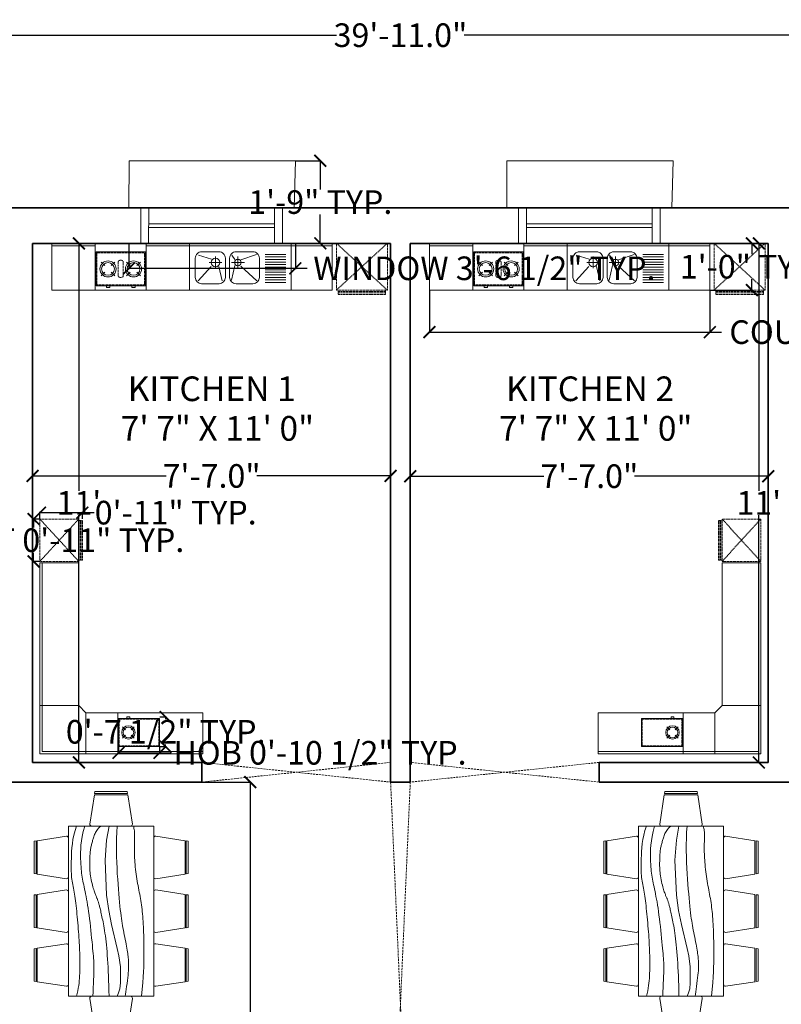
# Model space of a CAD drawing. Units: inches. Extents: x 844 to 2234, y 346 to 1084.
# Tile 92 of 93: x 1840 to 2033, y 828 to 1078. Entities that reach past the tile are written whole.
import ezdxf

# ---------------------------------------------------------------- set-up
doc = ezdxf.new("R2010")
doc.units = ezdxf.units.IN
doc.header["$MEASUREMENT"] = 0
doc.linetypes.add('DASHED', pattern=[0.75, 0.5, -0.25])
doc.linetypes.add('HIDDEN', pattern=[0.375, 0.25, -0.125])
for name, color, linetype, lineweight in [('A-ANNO-DIMS', 2, 'Continuous', 18), ('A-AREA-IDEN', 7, 'Continuous', 18), ('A-EQPM', 42, 'Continuous', 18), ('A-EQPM-HIDN', 42, 'HIDDEN', 13), ('A-FLOR-CASE', 42, 'Continuous', 18), ('A-FLOR-FIXT', 8, 'Continuous', 18), ('A-WALL', 7, 'Continuous', 35), ('A-WALL-OVHD', 7, 'DASHED', 18), ('furniture', 8, 'Continuous', 18), ('windows', 1, 'Continuous', 18)]:
    doc.layers.add(name, color=color, linetype=linetype, lineweight=lineweight)
doc.styles.add('ATTR', font='romans.shx', dxfattribs={"width": 0.8, "height": 0.7})
doc.styles.get("Standard").update_dxf_attribs({"font": 'arial.ttf'})
doc.dimstyles.get("Standard").update_dxf_attribs({"dimtxt": 6, "dimasz": 3, "dimexe": 0.18, "dimexo": 0.0625, "dimgap": 0.09, "dimtad": 0, "dimtih": 1, "dimtoh": 1, "dimdec": 1, "dimzin": 0, "dimdsep": 46, "dimlunit": 3, "dimtxsty": 'Standard', "dimblk": 'ARCHTICK', "dimcen": 0.09, "dimadec": 0, "dimazin": 0, "dimtfac": 1, "dimtdec": 1, "dimtofl": 0, "dimtmove": 0, "dimatfit": 3, "dimfxl": 1, "dimtolj": 1, "dimtzin": 0, "dimarcsym": 0})

# ---------------------------------------------------------------- blocks, each defined once
blk = doc.blocks.new('DIN42X84')
for p, q in [((-34.772, 36.500609), (-37.0377, 21.999999)), ((-34.7681, 36.499999), (-18.2986, 36.499999)), ((-34.5377, 37.999999), (-34.6939, 37.000439)), ((-18.3793, 36.999999), (-34.6911, 36.999999)), ((-34.5377, 37.999999), (-18.5377, 37.999999)), ((-18.3814, 36.999659), (-18.5377, 37.999999)), ((-16.0377, 21.999999), (-18.3032, 36.499269)), ((-8.2343, 36.500609), (-10.5001, 21.999999)), ((-8.2305, 36.499999), (8.2391, 36.499999)), ((-8.0001, 37.999999), (-8.1562, 37.000439)), ((8.1584, 36.999999), (-8.1535, 36.999999)), ((-8.0001, 37.999999), (7.9999, 37.999999)), ((8.1562, 36.999659), (7.9999, 37.999999)), ((10.4999, 21.999999), (8.2344, 36.499269)), ((16.0376, 21.999999), (18.3031, 36.499269)), ((34.768, 36.499999), (18.2985, 36.499999)), ((18.3792, 36.999999), (34.691, 36.999999)), ((18.3813, 36.999659), (18.5376, 37.999999)), ((34.5376, 37.999999), (18.5376, 37.999999)), ((34.5376, 37.999999), (34.6938, 37.000439)), ((34.7719, 36.500609), (37.0376, 21.999999)), ((-43, 10.499989), (-57.4993, 8.234489)), ((43, 10.499989), (57.4992, 8.234489)), ((-57.9997, 8.156299), (-59, 7.999989)), ((-59, -8.000011), (-59, 7.999989)), ((-58, 8.158429), (-58, -8.153391)), ((-57.5, -8.230411), (-57.5, 8.239139)), ((57.5, -8.230411), (57.5, 8.239139)), ((57.9996, 8.156299), (59, 7.999989)), ((58, 8.158429), (58, -8.153391)), ((59, -8.000011), (59, 7.999989)), ((-59, -8.000011), (-58.0005, -8.156181)), ((-57.5007, -8.234271), (-43, -10.500011)), ((57.5006, -8.234271), (43, -10.500011)), ((59, -8.000011), (58.0004, -8.156181)), ((-42, -21.000001), (42, -21.000001)), ((-34.772, -36.50061), (-37.0377, -22.000001)), ((-16.0377, -22.000001), (-18.3032, -36.499267)), ((-8.2343, -36.50061), (-10.5001, -22.000001)), ((10.4999, -22.000001), (8.2344, -36.499267)), ((16.0376, -22.000001), (18.3031, -36.499267)), ((34.7719, -36.50061), (37.0376, -22.000001)), ((-34.7681, -36.499999), (-18.2986, -36.499999)), ((-34.5377, -37.999999), (-34.6939, -37.000442)), ((-18.3793, -36.999999), (-34.6911, -36.999999)), ((-34.5377, -37.999999), (-18.5377, -37.999999)), ((-18.3814, -36.999664), (-18.5377, -37.999999)), ((-8.2305, -36.499999), (8.2391, -36.499999)), ((-8.0001, -37.999999), (-8.1562, -37.000442)), ((8.1584, -36.999999), (-8.1535, -36.999999)), ((-8.0001, -37.999999), (7.9999, -37.999999)), ((8.1562, -36.999664), (7.9999, -37.999999)), ((34.768, -36.499999), (18.2985, -36.499999)), ((18.3792, -36.999999), (34.691, -36.999999)), ((18.3813, -36.999664), (18.5376, -37.999999)), ((34.5376, -37.999999), (18.5376, -37.999999)), ((34.5376, -37.999999), (34.6938, -37.000442))]:
    blk.add_line(p, q)
for points in [[(-42, -21.000001), (-42, 20.999989), (42, 20.999989), (42, -21.000001)], [(-42, 16.999989), (-40.5974, 16.672209), (-39.2569, 16.395939), (-37.9668, 16.166109), (-36.7153, 15.977689), (-35.4906, 15.825599), (-34.281, 15.704799), (-33.0745, 15.610229), (-31.8595, 15.536839), (-30.6267, 15.480229), (-29.3778, 15.438619), (-28.117, 15.410889), (-26.8486, 15.395929), (-25.5767, 15.392599), (-24.3058, 15.399809), (-23.0399, 15.416409), (-21.7833, 15.441309), (-20.5384, 15.473619), (-19.2994, 15.513549), (-18.0587, 15.561549), (-16.8087, 15.618049), (-15.5417, 15.683499), (-14.25, 15.758369), (-12.9261, 15.843079), (-11.5622, 15.938089), (-10.1541, 16.043559), (-8.7108, 16.158419), (-7.2445, 16.281349), (-5.7675, 16.410999), (-4.2923, 16.546019), (-2.8311, 16.685069), (-1.3963, 16.826809), (0, 16.969889), (1.3474, 17.113339), (2.6447, 17.257689), (3.8928, 17.403829), (5.0924, 17.552659), (6.2444, 17.705069), (7.3498, 17.861959), (8.4092, 18.024219), (9.4237, 18.192759), (10.3952, 18.367629), (11.3311, 18.545639), (12.2397, 18.722759), (13.1297, 18.894949), (14.0095, 19.058179), (14.8876, 19.208429), (15.7725, 19.341659), (16.6727, 19.453839), (17.5977, 19.541909), (18.5617, 19.606689), (19.5795, 19.649979), (20.6664, 19.673569), (21.8374, 19.679239), (23.1076, 19.668789), (24.492, 19.644009), (26.0058, 19.606689), (27.6589, 19.554579), (29.4413, 19.469229), (31.3377, 19.328169), (33.3331, 19.108889), (35.4121, 18.788919), (37.5598, 18.345779), (39.7608, 17.756959), (42, 16.999989)], [(42, 12.999999), (39.3635, 13.704689), (36.9303, 14.232849), (34.6868, 14.608169), (32.6195, 14.854319), (30.7149, 14.994989), (28.9596, 15.053859), (27.34, 15.054629), (25.8427, 15.020959), (24.4543, 14.972439), (23.1628, 14.912279), (21.9562, 14.839589), (20.8227, 14.753449), (19.7504, 14.652989), (18.7273, 14.537299), (17.7416, 14.405489), (16.7814, 14.256669), (15.8348, 14.090369), (14.8899, 13.907959), (13.9348, 13.711209), (12.9575, 13.501929), (11.9464, 13.281899), (10.8893, 13.052909), (9.7745, 12.816759), (8.59, 12.575229), (7.3261, 12.330049), (5.9815, 12.082619), (4.557, 11.834299), (3.0536, 11.586429), (1.472, 11.340349), (-0.187, 11.097409), (-1.9223, 10.858939), (-3.7333, 10.626289), (-5.6141, 10.400739), (-7.539, 10.183249), (-9.4776, 9.974709), (-11.3991, 9.776019), (-13.2731, 9.588079), (-15.0689, 9.411789), (-16.756, 9.248039), (-18.3038, 9.097709), (-19.6928, 8.961719), (-20.9483, 8.840959), (-22.1065, 8.736319), (-23.2037, 8.648689), (-24.2763, 8.578979), (-25.3606, 8.528079), (-26.4928, 8.496879), (-27.7094, 8.486279), (-29.0411, 8.496689), (-30.4965, 8.526549), (-32.0787, 8.573829), (-33.7908, 8.636479), (-35.6359, 8.712459), (-37.6171, 8.799739), (-39.7374, 8.896259), (-42, 8.999999)], [(-42, 0.999999), (-39.2567, 1.059739), (-36.6668, 1.127399), (-34.2177, 1.203389), (-31.897, 1.288099), (-29.6923, 1.381949), (-27.5912, 1.485329), (-25.5812, 1.598659), (-23.65, 1.722319), (-21.7874, 1.856519), (-19.9935, 2.000569), (-18.2704, 2.153579), (-16.6207, 2.314649), (-15.0465, 2.482879), (-13.5503, 2.657379), (-12.1344, 2.837259), (-10.8011, 3.021619), (-9.5514, 3.209479), (-8.3812, 3.399579), (-7.2848, 3.590579), (-6.2569, 3.781129), (-5.2918, 3.969889), (-4.384, 4.155509), (-3.5281, 4.336659), (-2.7184, 4.511979), (-1.9505, 4.680359), (-1.2233, 4.841579), (-0.5369, 4.995629), (0.1087, 5.142519), (0.7135, 5.282239), (1.2776, 5.414799), (1.8009, 5.540189), (2.2834, 5.658409), (2.7259, 5.769699), (3.1323, 5.875159), (3.5073, 5.976139), (3.8555, 6.073989), (4.1816, 6.170049), (4.4904, 6.265659), (4.7863, 6.362169), (5.0742, 6.460919), (5.3584, 6.563099), (5.6417, 6.669299), (5.9267, 6.779989), (6.216, 6.895609), (6.512, 7.016589), (6.8174, 7.143399), (7.1347, 7.276479), (7.4664, 7.416279), (7.8159, 7.563169), (8.1896, 7.717219), (8.5948, 7.878439), (9.0386, 8.046819), (9.5282, 8.222369), (10.071, 8.405079), (10.674, 8.594959), (11.3446, 8.791999), (12.0866, 8.995459), (12.8902, 9.201609), (13.7421, 9.405969), (14.6294, 9.604059), (15.5387, 9.791399), (16.4569, 9.963509), (17.3709, 10.115919), (18.2674, 10.244149), (19.1361, 10.344989), (19.9772, 10.420299), (20.7936, 10.473209), (21.5884, 10.506879), (22.3645, 10.524419), (23.1248, 10.528969), (23.8725, 10.523669), (24.6103, 10.511649), (25.3403, 10.495379), (26.0601, 10.474629), (26.7663, 10.448509), (27.4556, 10.416119), (28.1244, 10.376559), (28.7695, 10.328939), (29.3873, 10.272359), (29.9746, 10.205939), (30.5293, 10.129059), (31.0552, 10.042329), (31.5572, 9.946639), (32.0406, 9.842899), (32.5104, 9.731989), (32.9716, 9.614799), (33.4295, 9.492249), (33.8891, 9.365219), (34.3546, 9.234229), (34.8266, 9.098309), (35.3051, 8.956129), (35.7897, 8.806329), (36.2802, 8.647569), (36.7765, 8.478519), (37.2783, 8.297819), (37.7854, 8.104139), (38.2976, 7.894309), (38.8146, 7.657969), (39.3361, 7.382899), (39.8617, 7.056919), (40.3912, 6.667829), (40.9243, 6.203449), (41.4607, 5.651569), (42, 4.999999)], [(42, 0.999999), (35.1214, 2.295539), (25.1178, 2.983399), (7.9376, 2.295539), (0.3261, 1.149099), (-6.6329, -0.226611), (-18.3763, -2.978061), (-22.0733, -3.895201), (-27.5101, -4.583071), (-32.9468, -4.583071), (-35.339, -4.583071), (-38.3836, -4.353771), (-40.3408, -3.665921), (-42, -3.000001)], [(42, -3.000001), (38.9344, -2.781351), (35.8829, -2.650251), (32.8567, -2.595491), (29.8672, -2.605821), (26.9257, -2.670031), (24.0436, -2.776881), (21.2323, -2.915141), (18.5031, -3.073591), (15.8668, -3.242611), (13.3327, -3.419021), (10.9095, -3.601241), (8.6059, -3.787731), (6.4305, -3.976901), (4.3921, -4.167191), (2.4994, -4.357031), (0.7611, -4.544851), (-0.8196, -4.729651), (-2.2614, -4.912671), (-3.5885, -5.095681), (-4.8252, -5.280481), (-5.9956, -5.468861), (-7.1239, -5.662621), (-8.2344, -5.863551), (-9.3513, -6.073431), (-10.4925, -6.293091), (-11.6511, -6.519461), (-12.814, -6.748531), (-13.968, -6.976251), (-15.0999, -7.198591), (-16.1965, -7.411531), (-17.2447, -7.611041), (-18.2313, -7.793081), (-19.1472, -7.954521), (-19.9994, -8.095811), (-20.7989, -8.218291), (-21.5568, -8.323311), (-22.2841, -8.412201), (-22.9919, -8.486311), (-23.6912, -8.546991), (-24.393, -8.595581), (-25.1087, -8.632751), (-25.8513, -8.656491), (-26.6337, -8.664101), (-27.4693, -8.652901), (-28.3711, -8.620211), (-29.3523, -8.563341), (-30.4262, -8.479601), (-31.6057, -8.366301), (-32.8956, -8.222561), (-34.2657, -8.054761), (-35.6772, -7.871051), (-37.0913, -7.679611), (-38.4695, -7.488621), (-39.7728, -7.306241), (-40.9626, -7.140641), (-42, -7.000001)], [(-42, -15.000001), (-38.4722, -15.350691), (-35.3039, -15.623741), (-32.4544, -15.828971), (-29.8831, -15.976191), (-27.5493, -16.075201), (-25.4123, -16.135831), (-23.4313, -16.167881), (-21.5659, -16.181151), (-19.7812, -16.183881), (-18.0665, -16.177871), (-16.4173, -16.163351), (-14.8288, -16.140551), (-13.2964, -16.109691), (-11.8154, -16.070991), (-10.3811, -16.024671), (-8.9888, -15.970971), (-7.6345, -15.909991), (-6.3163, -15.841401), (-5.0329, -15.764751), (-3.7831, -15.679591), (-2.5656, -15.585471), (-1.3791, -15.481951), (-0.2223, -15.368571), (0.9061, -15.244901), (2.0079, -15.110631), (3.0876, -14.966051), (4.1503, -14.811631), (5.2011, -14.647801), (6.2451, -14.475011), (7.2875, -14.293721), (8.3332, -14.104361), (9.3874, -13.907391), (10.4544, -13.703711), (11.5349, -13.495991), (12.6291, -13.287381), (13.7368, -13.081011), (14.8581, -12.880011), (15.9931, -12.687521), (17.1416, -12.506671), (18.3037, -12.340601), (19.4778, -12.191771), (20.6562, -12.059961), (21.8295, -11.944271), (22.9884, -11.843811), (24.1234, -11.757681), (25.2254, -11.684981), (26.2848, -11.624831), (27.2925, -11.576311), (28.2412, -11.538551), (29.1325, -11.510631), (29.9703, -11.491671), (30.7584, -11.480781), (31.5007, -11.477041), (32.2009, -11.479581), (32.8628, -11.487491), (33.4904, -11.499881), (34.0874, -11.515741), (34.6576, -11.533621), (35.2049, -11.551941), (35.733, -11.569151), (36.2459, -11.583661), (36.7473, -11.593931), (37.2411, -11.598371), (37.7311, -11.595421), (38.2211, -11.583281), (38.7152, -11.559251), (39.2177, -11.520361), (39.7326, -11.463671), (40.2641, -11.386241), (40.8164, -11.285111), (41.3937, -11.157351), (42, -11.000001)]]:
    blk.add_lwpolyline(points)
for centre, start, end in [((-36.0377, 21.999999), 180, 270), ((-17.0377, 21.999999), 270, 0), ((-9.5001, 21.999999), 180, 270), ((9.4999, 21.999999), 270, 0), ((17.0376, 21.999999), 180, 270), ((36.0376, 21.999999), 270, 0), ((-43, 9.499989), 0.00000068, 90), ((43, 9.499989), 90, 180), ((-43, -9.500011), 270, 0.00000068), ((43, -9.500011), 180, 270), ((-36.0377, -22.000001), 90, 180), ((-17.0377, -22.000001), 0, 90), ((-9.5001, -22.000001), 90, 180), ((9.4999, -22.000001), 0, 90), ((17.0376, -22.000001), 90, 180), ((36.0376, -22.000001), 0, 90)]:
    blk.add_arc(centre, 1, start, end)
at = {"style": 'ATTR', "width": 0.8, "flags": 9}
blk.add_attdef('ESTCODE', (0, 0), '', height=0.7, dxfattribs=at)
blk = doc.blocks.new('_ArchTick')
at = {"color": 0, "linetype": 'ByBlock', "const_width": 0.15}
blk.add_lwpolyline([(-0.5, -0.5), (0.5, 0.5)], dxfattribs=at)
blk = doc.blocks.new('*D90')
at = {"layer": 'A-ANNO-DIMS', "color": 0, "lineweight": -2, "transparency": 16777216}
for p, q in [((1843.1, 962.31), (1877.06, 962.31)), ((1843.1, 962.25), (1843.1, 962.13)), ((1934.1, 962.31), (1900.13, 962.31)), ((1934.1, 962.37), (1934.1, 962.49))]:
    blk.add_line(p, q, dxfattribs=at)
at = {"layer": 'Defpoints', "color": 0, "transparency": 16777216}
for p in [(1843.1, 962.31), (1934.1, 962.31), (1934.1, 962.31)]:
    blk.add_point(p, dxfattribs=at)
at = {"layer": 'A-ANNO-DIMS', "color": 0, "lineweight": -2, "transparency": 16777216, "xscale": 3, "yscale": 3, "zscale": 3, "rotation": 180}
blk.add_blockref('_ArchTick', (1843.1, 962.31), dxfattribs=at)
at = {"layer": 'A-ANNO-DIMS', "color": 0, "lineweight": -2, "transparency": 16777216, "xscale": 3, "yscale": 3, "zscale": 3}
blk.add_blockref('_ArchTick', (1934.1, 962.31), dxfattribs=at)
at = {"layer": 'A-ANNO-DIMS', "color": 0, "transparency": 16777216, "insert": (1888.6, 962.31), "char_height": 6, "attachment_point": 5}
blk.add_mtext('\\A1;7\'-7.0"', dxfattribs=at)
blk = doc.blocks.new('*D57')
at = {"layer": 'A-ANNO-DIMS', "color": 0, "lineweight": -2, "transparency": 16777216}
for p, q in [((1846.19, 1021.46), (1855.04, 1021.46)), ((1854.86, 1021.46), (1854.86, 958.56)), ((1854.86, 889.46), (1854.86, 952.35)), ((1846.19, 889.46), (1855.04, 889.46))]:
    blk.add_line(p, q, dxfattribs=at)
at = {"layer": 'Defpoints', "color": 0, "transparency": 16777216}
for p in [(1846.12, 1021.46), (1846.12, 889.46), (1854.86, 889.46)]:
    blk.add_point(p, dxfattribs=at)
at = {"layer": 'A-ANNO-DIMS', "color": 0, "lineweight": -2, "transparency": 16777216, "xscale": 3, "yscale": 3, "zscale": 3}
for p, rotation in [((1854.86, 1021.46), 90), ((1854.86, 889.46), 270)]:
    blk.add_blockref('_ArchTick', p, dxfattribs=dict(at, rotation=rotation))
at = {"layer": 'A-ANNO-DIMS', "color": 0, "transparency": 16777216, "insert": (1854.86, 955.46), "char_height": 6, "attachment_point": 5}
blk.add_mtext("\\A1;11'", dxfattribs=at)
blk = doc.blocks.new('*D58')
at = {"layer": 'A-ANNO-DIMS', "color": 0, "lineweight": -2, "transparency": 16777216}
for p, q in [((2029.69, 1021.46), (2027.51, 1021.46)), ((2027.69, 1021.46), (2027.69, 958.56)), ((2027.69, 889.46), (2027.69, 952.35)), ((2029.69, 889.46), (2027.51, 889.46))]:
    blk.add_line(p, q, dxfattribs=at)
at = {"layer": 'Defpoints', "color": 0, "transparency": 16777216}
for p in [(2029.76, 1021.46), (2027.69, 889.46), (2029.76, 889.46)]:
    blk.add_point(p, dxfattribs=at)
at = {"layer": 'A-ANNO-DIMS', "color": 0, "lineweight": -2, "transparency": 16777216, "xscale": 3, "yscale": 3, "zscale": 3}
for p, rotation in [((2027.69, 1021.46), 90), ((2027.69, 889.46), 270)]:
    blk.add_blockref('_ArchTick', p, dxfattribs=dict(at, rotation=rotation))
at = {"layer": 'A-ANNO-DIMS', "color": 0, "transparency": 16777216, "insert": (2027.69, 955.46), "char_height": 6, "attachment_point": 5}
blk.add_mtext("\\A1;11'", dxfattribs=at)
blk = doc.blocks.new('*D59')
at = {"layer": 'A-ANNO-DIMS', "color": 0, "lineweight": -2, "transparency": 16777216}
for p, q in [((1939.1, 962.31), (1939.1, 962.43)), ((1939.1, 962.25), (1973.06, 962.25)), ((2030.1, 962.25), (1996.13, 962.25)), ((2030.1, 962.31), (2030.1, 962.43))]:
    blk.add_line(p, q, dxfattribs=at)
at = {"layer": 'Defpoints', "color": 0, "transparency": 16777216}
for p in [(1939.1, 962.25), (2030.1, 962.25), (2030.1, 962.25)]:
    blk.add_point(p, dxfattribs=at)
at = {"layer": 'A-ANNO-DIMS', "color": 0, "lineweight": -2, "transparency": 16777216, "xscale": 3, "yscale": 3, "zscale": 3, "rotation": 180}
blk.add_blockref('_ArchTick', (1939.1, 962.25), dxfattribs=at)
at = {"layer": 'A-ANNO-DIMS', "color": 0, "lineweight": -2, "transparency": 16777216, "xscale": 3, "yscale": 3, "zscale": 3}
blk.add_blockref('_ArchTick', (2030.1, 962.25), dxfattribs=at)
at = {"layer": 'A-ANNO-DIMS', "color": 0, "transparency": 16777216, "insert": (1984.6, 962.25), "char_height": 6, "attachment_point": 5}
blk.add_mtext('\\A1;7\'-7.0"', dxfattribs=at)
blk = doc.blocks.new('*D85')
at = {"layer": 'A-ANNO-DIMS', "color": 0, "lineweight": -2, "transparency": 16777216}
for p, q in [((1886.16, 884.46), (1898.6, 884.46)), ((1898.42, 884.46), (1898.42, 763.55)), ((1898.42, 636.33), (1898.42, 757.24)), ((1886.16, 636.33), (1898.6, 636.33))]:
    blk.add_line(p, q, dxfattribs=at)
at = {"layer": 'Defpoints', "color": 0, "transparency": 16777216}
for p in [(1886.1, 884.46), (1886.1, 636.33), (1898.42, 636.33)]:
    blk.add_point(p, dxfattribs=at)
at = {"layer": 'A-ANNO-DIMS', "color": 0, "lineweight": -2, "transparency": 16777216, "xscale": 3, "yscale": 3, "zscale": 3}
for p, rotation in [((1898.42, 884.46), 90), ((1898.42, 636.33), 270)]:
    blk.add_blockref('_ArchTick', p, dxfattribs=dict(at, rotation=rotation))
at = {"layer": 'A-ANNO-DIMS', "color": 0, "transparency": 16777216, "insert": (1898.42, 760.39), "char_height": 6, "attachment_point": 5}
blk.add_mtext('\\A1;20\'-8.1"', dxfattribs=at)
blk = doc.blocks.new('*D86')
at = {"layer": 'A-ANNO-DIMS', "color": 0, "lineweight": -2, "transparency": 16777216}
for p, q in [((1697.1, 1030.52), (1697.1, 1074.57)), ((1697.1, 1074.39), (1920.38, 1074.39)), ((2176.1, 1074.39), (1952.82, 1074.39)), ((2176.1, 1030.52), (2176.1, 1074.57))]:
    blk.add_line(p, q, dxfattribs=at)
at = {"layer": 'Defpoints', "color": 0, "transparency": 16777216}
for p in [(2176.1, 1074.39), (1697.1, 1030.46), (2176.1, 1030.46)]:
    blk.add_point(p, dxfattribs=at)
at = {"layer": 'A-ANNO-DIMS', "color": 0, "lineweight": -2, "transparency": 16777216, "xscale": 3, "yscale": 3, "zscale": 3, "rotation": 180}
blk.add_blockref('_ArchTick', (1697.1, 1074.39), dxfattribs=at)
at = {"layer": 'A-ANNO-DIMS', "color": 0, "lineweight": -2, "transparency": 16777216, "xscale": 3, "yscale": 3, "zscale": 3}
blk.add_blockref('_ArchTick', (2176.1, 1074.39), dxfattribs=at)
at = {"layer": 'A-ANNO-DIMS', "color": 0, "transparency": 16777216, "insert": (1936.6, 1074.39), "char_height": 6, "attachment_point": 5}
blk.add_mtext('\\A1;39\'-11.0"', dxfattribs=at)
blk = doc.blocks.new('WIN-36IN')
for p, q in [((0, 9), (0, 21)), ((0, 21), (42.29, 21)), ((42, 9), (42.29, 21)), ((3, 9), (0, 9)), ((39, 9), (3, 9)), ((3, 9), (3, 0)), ((5, 9), (5, 0)), ((37, 0), (37, 9)), ((39, 0), (39, 9)), ((39, 9), (42, 9)), ((5, 5), (37, 5)), ((5, 4), (37, 4)), ((3, 0), (39, 0))]:
    blk.add_line(p, q)
blk = doc.blocks.new('KITCHEN-TALL-UNIT')
for p, q in [((12.96, 1.08), (0, 12.96)), ((0, 1.08), (12.96, 12.96)), ((0.43, 0.73), (12.53, 0.73)), ((0.43, 0.37), (12.53, 0.37))]:
    blk.add_line(p, q)
blk.add_lwpolyline([(0, 1.08), (0, 12.96), (12.96, 12.96), (12.96, 1.08)], close=True)
blk.add_lwpolyline([(0.43, 1.08), (0.43, 0), (12.53, 0), (12.53, 1.08)])
blk = doc.blocks.new('KITCHEN-TALL-UNIT-COMPACT')
for p, q in [((9.89, 0), (0, 10.79)), ((9.89, 10.79), (0, 0)), ((10.18, 0.36), (10.18, 10.43)), ((10.48, 0.36), (10.48, 10.43))]:
    blk.add_line(p, q)
blk.add_lwpolyline([(9.89, 0), (0, 0), (0, 10.79), (9.89, 10.79)], close=True)
blk.add_lwpolyline([(9.89, 0.36), (10.79, 0.36), (10.79, 10.43), (9.89, 10.43)])
blk = doc.blocks.new('KITCHEN-COUNTER-LINEAR')
for p, q in [((0, 11.88), (34.99, 11.88)), ((0, 11.88), (0, 0)), ((0, 11.23), (11.08, 11.23)), ((11.08, 11.88), (11.08, 0)), ((24.04, 11.88), (24.04, 0)), ((24.04, 11.23), (34.99, 11.23)), ((34.99, 11.23), (60.91, 11.23)), ((60.91, 11.88), (71.28, 11.88)), ((60.91, 11.23), (71.28, 11.23)), ((71.28, 11.88), (71.28, 0)), ((0, 0), (34.99, 0)), ((60.91, 0), (71.28, 0))]:
    blk.add_line(p, q)
blk = doc.blocks.new('KITCHEN-COUNTER-L')
for p, q in [((0, 0), (0, 48.56)), ((0, 48.56), (9.89, 48.56)), ((0.54, 0.54), (0.54, 48.56)), ((9.89, 12.23), (9.89, 48.56)), ((9.89, 12.23), (0, 12.23)), ((11.69, 10.43), (9.89, 12.23)), ((11.69, 10.43), (11.69, 0)), ((11.69, 10.43), (41.36, 10.43)), ((19.78, 0), (19.78, 10.43)), ((41.36, 0), (41.36, 10.43)), ((0.54, 0.54), (41.36, 0.54)), ((0, 0), (41.36, 0)), ((0, 0), (9.89, 0))]:
    blk.add_line(p, q)
blk = doc.blocks.new('HOB-2-BURNER')
for p, q in [((1.27, 6.49), (2.18, 5.57)), ((3.86, 5.57), (4.78, 6.49)), ((7.75, 6.49), (8.66, 5.57)), ((10.34, 5.57), (11.26, 6.49)), ((1.27, 2.97), (2.18, 3.89)), ((3.86, 3.89), (4.78, 2.97)), ((7.75, 2.97), (8.66, 3.89)), ((10.34, 3.89), (11.26, 2.97))]:
    blk.add_line(p, q)
blk.add_lwpolyline([(0, 9.07), (0, 0.43), (12.53, 0.43), (12.53, 9.07)], close=True)
for points in [[(2.59, 0.43), (2.59, 0), (3.46, 0), (3.46, 0.45)], [(9.07, 0.43), (9.07, 0), (9.94, 0), (9.94, 0.45)]]:
    blk.add_lwpolyline(points)
for centre, radius in [((3.02, 4.73), 2.05), ((3.02, 4.73), 1.62), ((9.5, 4.73), 2.05), ((9.5, 4.73), 1.62)]:
    blk.add_circle(centre, radius)
blk = doc.blocks.new('HOB-1-BURNER')
for p, q in [((1.82, 4.31), (1.06, 5.08)), ((3.98, 5.08), (3.22, 4.31)), ((1.82, 2.92), (1.06, 2.15)), ((3.98, 2.15), (3.22, 2.92))]:
    blk.add_line(p, q)
blk.add_lwpolyline([(2.88, 7.19), (2.88, 7.55), (2.16, 7.55), (2.16, 7.18)])
blk.add_lwpolyline([(10.43, 0), (10.43, 7.19), (0, 7.19), (0, 0)], close=True)
for radius in [1.71, 1.35]:
    blk.add_circle((2.52, 3.61), radius)
blk = doc.blocks.new('SINK-DOUBLE-DRAINBOARD')
for p, q in [((5.62, 7.84), (2.31, 8.86)), ((6.65, 5.57), (6.65, 8.58)), ((11.53, 7.78), (10.82, 8.86)), ((12.33, 5.55), (12.33, 8.55)), ((13.11, 7.71), (17.09, 9.07)), ((19.31, 9.07), (24.52, 9.07)), ((19.31, 8.42), (24.52, 8.42)), ((19.31, 7.78), (24.52, 7.78)), ((2.23, 2.35), (5.55, 5.96)), ((5.05, 7.02), (8.29, 7.02)), ((8.36, 2.35), (7.5, 5.96)), ((10.74, 7), (13.98, 7)), ((11.53, 6.26), (10.74, 2.51)), ((13.11, 6.11), (17.15, 2.35)), ((19.31, 7.13), (24.52, 7.13)), ((19.31, 6.48), (24.52, 6.48)), ((19.31, 5.83), (24.52, 5.83)), ((19.31, 5.18), (24.52, 5.18)), ((19.31, 4.54), (24.52, 4.54)), ((19.31, 3.89), (24.52, 3.89)), ((19.31, 3.24), (24.52, 3.24)), ((19.31, 2.59), (24.52, 2.59)), ((19.31, 1.94), (24.52, 1.94))]:
    blk.add_line(p, q)
blk.add_lwpolyline([(0, 0), (25.92, 0), (25.92, 11.88), (0, 11.88)], close=True)
for points in [[(1.51, 8.1), (1.51, 3.24, 0.414214), (3.13, 1.62), (7.54, 1.62, 0.414214), (9.16, 3.24), (9.16, 8.1, 0.414214), (7.54, 9.72), (3.13, 9.72, 0.414214)], [(10.24, 8.1), (10.24, 3.24, 0.414214), (11.86, 1.62), (16.18, 1.62, 0.414214), (17.8, 3.24), (17.8, 8.1, 0.414214), (16.18, 9.72), (11.86, 9.72, 0.414214)]]:
    blk.add_lwpolyline(points, format="xyb", close=True)
for centre, radius in [((6.65, 7.02), 1.08), ((12.33, 7), 0.81)]:
    blk.add_circle(centre, radius)
blk = doc.blocks.new('*D123')
at = {"layer": 'A-ANNO-DIMS', "color": 0, "lineweight": -2, "transparency": 16777216}
for p, q in [((1867.6, 1021.4), (1867.6, 1014.93)), ((1909.89, 1021.39), (1909.89, 1014.93)), ((1867.6, 1015.11), (1909.89, 1015.11)), ((1909.89, 1015.11), (1912.89, 1015.11))]:
    blk.add_line(p, q, dxfattribs=at)
at = {"layer": 'Defpoints', "color": 0, "transparency": 16777216}
for p in [(1867.6, 1021.46), (1909.89, 1021.45), (1909.89, 1015.11)]:
    blk.add_point(p, dxfattribs=at)
at = {"layer": 'A-ANNO-DIMS', "color": 0, "lineweight": -2, "transparency": 16777216, "xscale": 3, "yscale": 3, "zscale": 3}
for p, rotation in [((1867.6, 1015.11), 179.9931124012453), ((1909.89, 1015.11), 359.9931124012453)]:
    blk.add_blockref('_ArchTick', p, dxfattribs=dict(at, rotation=rotation))
at = {"layer": 'A-ANNO-DIMS', "color": 0, "transparency": 16777216, "insert": (1957.93, 1015.11), "char_height": 6, "attachment_point": 5}
blk.add_mtext('\\A1;WINDOW 3\'-6 1/2" TYP.', dxfattribs=at)
blk = doc.blocks.new('*D124')
at = {"layer": 'A-ANNO-DIMS', "color": 0, "lineweight": -2, "transparency": 16777216}
for p, q in [((1909.95, 1042.45), (1916.41, 1042.45)), ((1916.23, 1042.45), (1916.23, 1035.11)), ((1916.23, 1021.45), (1916.23, 1028.8)), ((1909.95, 1021.45), (1916.41, 1021.45))]:
    blk.add_line(p, q, dxfattribs=at)
at = {"layer": 'Defpoints', "color": 0, "transparency": 16777216}
for p in [(1909.89, 1042.45), (1916.23, 1042.45), (1909.89, 1021.45)]:
    blk.add_point(p, dxfattribs=at)
at = {"layer": 'A-ANNO-DIMS', "color": 0, "lineweight": -2, "transparency": 16777216, "xscale": 3, "yscale": 3, "zscale": 3}
for p, rotation in [((1916.23, 1042.45), 89.99311240124487), ((1916.23, 1021.45), 269.9931124012449)]:
    blk.add_blockref('_ArchTick', p, dxfattribs=dict(at, rotation=rotation))
at = {"layer": 'A-ANNO-DIMS', "color": 0, "transparency": 16777216, "insert": (1916.23, 1031.95), "char_height": 6, "attachment_point": 5}
blk.add_mtext('\\A1;1\'-9" TYP.', dxfattribs=at)
blk = doc.blocks.new('*D127')
at = {"layer": 'A-ANNO-DIMS', "color": 0, "lineweight": -2, "transparency": 16777216}
for p, q in [((1844.9, 951.36), (1843.17, 951.36)), ((1843.35, 951.36), (1843.35, 949.16)), ((1843.35, 940.57), (1843.35, 942.78)), ((1844.9, 940.57), (1843.17, 940.57))]:
    blk.add_line(p, q, dxfattribs=at)
at = {"layer": 'Defpoints', "color": 0, "transparency": 16777216}
for p in [(1843.35, 951.36), (1844.97, 951.36), (1844.97, 940.57)]:
    blk.add_point(p, dxfattribs=at)
at = {"layer": 'A-ANNO-DIMS', "color": 0, "lineweight": -2, "transparency": 16777216, "xscale": 3, "yscale": 3, "zscale": 3}
for p, rotation in [((1843.35, 951.36), 90), ((1843.35, 940.57), 270)]:
    blk.add_blockref('_ArchTick', p, dxfattribs=dict(at, rotation=rotation))
at = {"layer": 'A-ANNO-DIMS', "color": 0, "transparency": 16777216, "insert": (1843.35, 945.97), "char_height": 6, "attachment_point": 5}
blk.add_mtext('\\A1;CABINET 0\'-11" TYP.', dxfattribs=at)
blk = doc.blocks.new('*D128')
at = {"layer": 'A-ANNO-DIMS', "color": 0, "lineweight": -2, "transparency": 16777216}
for p, q in [((1844.97, 951.43), (1844.97, 953.16)), ((1844.97, 952.98), (1855.76, 952.98)), ((1855.76, 951.43), (1855.76, 953.16)), ((1855.76, 952.98), (1858.76, 952.98))]:
    blk.add_line(p, q, dxfattribs=at)
at = {"layer": 'Defpoints', "color": 0, "transparency": 16777216}
for p in [(1855.76, 952.98), (1844.97, 951.36), (1855.76, 951.36)]:
    blk.add_point(p, dxfattribs=at)
at = {"layer": 'A-ANNO-DIMS', "color": 0, "lineweight": -2, "transparency": 16777216, "xscale": 3, "yscale": 3, "zscale": 3, "rotation": 180}
blk.add_blockref('_ArchTick', (1844.97, 952.98), dxfattribs=at)
at = {"layer": 'A-ANNO-DIMS', "color": 0, "lineweight": -2, "transparency": 16777216, "xscale": 3, "yscale": 3, "zscale": 3}
blk.add_blockref('_ArchTick', (1855.76, 952.98), dxfattribs=at)
at = {"layer": 'A-ANNO-DIMS', "color": 0, "transparency": 16777216, "insert": (1879.47, 952.98), "char_height": 6, "attachment_point": 5}
blk.add_mtext('\\A1;0\'-11" TYP.', dxfattribs=at)
blk = doc.blocks.new('*D129')
at = {"layer": 'A-ANNO-DIMS', "color": 0, "lineweight": -2, "transparency": 16777216}
for p, q in [((1943.95, 1009.51), (1943.95, 998.7)), ((2015.23, 1009.51), (2015.23, 998.7)), ((1943.95, 998.88), (2015.23, 998.88)), ((2015.23, 998.88), (2018.23, 998.88))]:
    blk.add_line(p, q, dxfattribs=at)
at = {"layer": 'Defpoints', "color": 0, "transparency": 16777216}
for p in [(1943.95, 1009.57), (2015.23, 1009.57), (2015.23, 998.88)]:
    blk.add_point(p, dxfattribs=at)
at = {"layer": 'A-ANNO-DIMS', "color": 0, "lineweight": -2, "transparency": 16777216, "xscale": 3, "yscale": 3, "zscale": 3, "rotation": 180}
blk.add_blockref('_ArchTick', (1943.95, 998.88), dxfattribs=at)
at = {"layer": 'A-ANNO-DIMS', "color": 0, "lineweight": -2, "transparency": 16777216, "xscale": 3, "yscale": 3, "zscale": 3}
blk.add_blockref('_ArchTick', (2015.23, 998.88), dxfattribs=at)
at = {"layer": 'A-ANNO-DIMS', "color": 0, "transparency": 16777216, "insert": (2067.78, 998.88), "char_height": 6, "attachment_point": 5}
blk.add_mtext('\\A1;COUNTER 5\'-11 1/2" TYP.', dxfattribs=at)
blk = doc.blocks.new('*D130')
at = {"layer": 'A-ANNO-DIMS', "color": 0, "lineweight": -2, "transparency": 16777216}
for p, q in [((2015.29, 1021.46), (2026.1, 1021.46)), ((2025.92, 1021.46), (2025.92, 1018.67)), ((2025.92, 1009.57), (2025.92, 1012.36)), ((2015.29, 1009.57), (2026.1, 1009.57))]:
    blk.add_line(p, q, dxfattribs=at)
at = {"layer": 'Defpoints', "color": 0, "transparency": 16777216}
for p in [(2015.23, 1021.46), (2025.92, 1021.46), (2015.23, 1009.57)]:
    blk.add_point(p, dxfattribs=at)
at = {"layer": 'A-ANNO-DIMS', "color": 0, "lineweight": -2, "transparency": 16777216, "xscale": 3, "yscale": 3, "zscale": 3}
for p, rotation in [((2025.92, 1021.46), 90), ((2025.92, 1009.57), 270)]:
    blk.add_blockref('_ArchTick', p, dxfattribs=dict(at, rotation=rotation))
at = {"layer": 'A-ANNO-DIMS', "color": 0, "transparency": 16777216, "insert": (2025.92, 1015.51), "char_height": 6, "attachment_point": 5}
blk.add_mtext('\\A1;1\'-0" TYP.', dxfattribs=at)
blk = doc.blocks.new('*D135')
at = {"layer": 'A-ANNO-DIMS', "color": 0, "lineweight": -2, "transparency": 16777216}
for p, q in [((1864.93, 893.41), (1864.93, 891.73)), ((1864.93, 891.91), (1875.36, 891.91)), ((1875.36, 893.41), (1875.36, 891.73)), ((1875.36, 891.91), (1878.36, 891.91))]:
    blk.add_line(p, q, dxfattribs=at)
at = {"layer": 'Defpoints', "color": 0, "transparency": 16777216}
for p in [(1864.93, 893.47), (1875.36, 893.47), (1875.36, 891.91)]:
    blk.add_point(p, dxfattribs=at)
at = {"layer": 'A-ANNO-DIMS', "color": 0, "lineweight": -2, "transparency": 16777216, "xscale": 3, "yscale": 3, "zscale": 3, "rotation": 180}
blk.add_blockref('_ArchTick', (1864.93, 891.91), dxfattribs=at)
at = {"layer": 'A-ANNO-DIMS', "color": 0, "lineweight": -2, "transparency": 16777216, "xscale": 3, "yscale": 3, "zscale": 3}
blk.add_blockref('_ArchTick', (1875.36, 891.91), dxfattribs=at)
at = {"layer": 'A-ANNO-DIMS', "color": 0, "transparency": 16777216, "insert": (1916.14, 891.91), "char_height": 6, "attachment_point": 5}
blk.add_mtext('\\A1;HOB 0\'-10 1/2" TYP.', dxfattribs=at)
blk = doc.blocks.new('*D136')
at = {"layer": 'A-ANNO-DIMS', "color": 0, "lineweight": -2, "transparency": 16777216}
for p, q in [((1875.42, 901.03), (1877.1, 901.03)), ((1876.92, 901.03), (1876.92, 900.44)), ((1876.92, 893.47), (1876.92, 894.06)), ((1875.42, 893.47), (1877.1, 893.47))]:
    blk.add_line(p, q, dxfattribs=at)
at = {"layer": 'Defpoints', "color": 0, "transparency": 16777216}
for p in [(1875.36, 901.03), (1876.92, 901.03), (1875.36, 893.47)]:
    blk.add_point(p, dxfattribs=at)
at = {"layer": 'A-ANNO-DIMS', "color": 0, "lineweight": -2, "transparency": 16777216, "xscale": 3, "yscale": 3, "zscale": 3}
for p, rotation in [((1876.92, 901.03), 90), ((1876.92, 893.47), 270)]:
    blk.add_blockref('_ArchTick', p, dxfattribs=dict(at, rotation=rotation))
at = {"layer": 'A-ANNO-DIMS', "color": 0, "transparency": 16777216, "insert": (1876.92, 897.25), "char_height": 6, "attachment_point": 5}
blk.add_mtext('\\A1;0\'-7 1/2" TYP.', dxfattribs=at)

msp = doc.modelspace()

# ---------------------------------------------------------------- linework, layer by layer
at = {"layer": 'A-EQPM-HIDN'}
for points in [[(1859.46, 1019.08), (1859.46, 1010.87), (1871.56, 1010.87), (1871.56, 1019.08)], [(1955.46, 1019.08), (1955.46, 1010.87), (1967.56, 1010.87), (1967.56, 1019.08)], [(1875.18, 893.65), (1875.18, 900.49), (1865.11, 900.49), (1865.11, 893.65)], [(1998.02, 893.65), (1998.02, 900.49), (2008.09, 900.49), (2008.09, 893.65)]]:
    msp.add_lwpolyline(points, close=True, dxfattribs=at)
for points in [[(1864.86, 1016.7), (1864.86, 1013.25, 0.414214), (1865.29, 1012.81), (1865.73, 1012.81, 0.414214), (1866.16, 1013.25), (1866.16, 1016.7, 0.414214), (1865.73, 1017.14), (1865.29, 1017.14, 0.414214)], [(1960.86, 1016.7), (1960.86, 1013.25, 0.414214), (1961.29, 1012.81), (1961.73, 1012.81, 0.414214), (1962.16, 1013.25), (1962.16, 1016.7, 0.414214), (1961.73, 1017.14), (1961.29, 1017.14, 0.414214)]]:
    msp.add_lwpolyline(points, format="xyb", close=True, dxfattribs=at)
at = {"layer": 'A-FLOR-FIXT'}
for p, q in [((1888.56, 1017.42), (1885.25, 1018.43)), ((1888, 1016.6), (1891.24, 1016.6)), ((1889.59, 1015.15), (1889.59, 1018.15)), ((1893.68, 1016.57), (1896.92, 1016.57)), ((1894.48, 1017.35), (1893.76, 1018.43)), ((1895.28, 1015.13), (1895.28, 1018.13)), ((1896.05, 1017.29), (1900.03, 1018.65)), ((1902.25, 1018.65), (1907.46, 1018.65)), ((1902.25, 1018), (1907.46, 1018)), ((1902.25, 1017.35), (1907.46, 1017.35)), ((1902.25, 1016.7), (1907.46, 1016.7)), ((1885.17, 1011.93), (1888.49, 1015.54)), ((1891.3, 1011.93), (1890.44, 1015.54)), ((1894.48, 1015.84), (1893.68, 1012.08)), ((1896.05, 1015.69), (1900.09, 1011.93)), ((1902.25, 1016.05), (1907.46, 1016.05)), ((1902.25, 1015.41), (1907.46, 1015.41)), ((1902.25, 1014.76), (1907.46, 1014.76)), ((1902.25, 1014.11), (1907.46, 1014.11)), ((1902.25, 1013.46), (1907.46, 1013.46)), ((1902.25, 1012.81), (1907.46, 1012.81)), ((1902.25, 1012.17), (1907.46, 1012.17)), ((1902.25, 1011.52), (1907.46, 1011.52))]:
    msp.add_line(p, q, dxfattribs=at)
msp.add_lwpolyline([(1882.94, 1009.57), (1908.86, 1009.57), (1908.86, 1021.46), (1882.94, 1021.46)], close=True, dxfattribs=at)
for points in [[(1884.45, 1017.68), (1884.45, 1012.81, 0.414214), (1886.07, 1011.19), (1890.48, 1011.19, 0.414214), (1892.1, 1012.81), (1892.1, 1017.68, 0.414214), (1890.48, 1019.3), (1886.07, 1019.3, 0.414214)], [(1893.18, 1017.68), (1893.18, 1012.81, 0.414214), (1894.8, 1011.19), (1899.12, 1011.19, 0.414214), (1900.74, 1012.81), (1900.74, 1017.68, 0.414214), (1899.12, 1019.3), (1894.8, 1019.3, 0.414214)]]:
    msp.add_lwpolyline(points, format="xyb", close=True, dxfattribs=at)
for centre, radius in [((1889.59, 1016.6), 1.08), ((1895.28, 1016.57), 0.81)]:
    msp.add_circle(centre, radius, dxfattribs=at)
at = {"layer": 'A-WALL'}
for p, q in [((1697.1, 1030.46), (2176.1, 1030.46)), ((1843.1, 1021.46), (1843.1, 889.46)), ((1843.1, 1021.46), (1934.1, 1021.46)), ((1934.1, 1021.46), (1934.1, 889.46)), ((1939.1, 1021.46), (1939.1, 889.46)), ((1939.1, 1021.46), (2030.1, 1021.46)), ((2030.1, 1021.46), (2030.1, 889.46)), ((1843.1, 889.46), (1886.1, 889.46)), ((1886.1, 889.46), (1886.1, 884.46)), ((1934.1, 889.46), (1934.1, 884.46)), ((1939.1, 889.46), (1939.1, 884.46)), ((1987.1, 889.46), (2030.1, 889.46)), ((1987.1, 889.46), (1987.1, 884.46)), ((1834.1, 884.46), (1886.1, 884.46)), ((1934.1, 884.46), (1939.1, 884.46)), ((1987.1, 884.46), (2039.1, 884.46))]:
    msp.add_line(p, q, dxfattribs=at)
at = {"layer": 'A-WALL-OVHD'}
for p, q in [((1886.1, 889.46), (1934.1, 884.46)), ((1886.1, 884.46), (1934.1, 889.46)), ((1987.1, 889.46), (1939.1, 884.46)), ((1987.1, 884.46), (1939.1, 889.46)), ((1939.1, 771.46), (1934.1, 884.46)), ((1939.1, 884.46), (1934.1, 771.46))]:
    msp.add_line(p, q, dxfattribs=at)

# ---------------------------------------------------------------- block references
at = {"layer": 'A-EQPM'}
for name, p in [('HOB-2-BURNER', (1859.25, 1010.22)), ('HOB-2-BURNER', (1955.25, 1010.22)), ('HOB-1-BURNER', (1864.93, 893.47))]:
    msp.add_blockref(name, p, dxfattribs=at)
at = {"layer": 'A-EQPM', "extrusion": (0, 0, -1), "zscale": -1}
msp.add_blockref('HOB-1-BURNER', (-2008.27, 893.47), dxfattribs=at)
at = {"layer": 'A-EQPM-HIDN'}
for name, p in [('KITCHEN-TALL-UNIT', (1920.31, 1008.49)), ('KITCHEN-TALL-UNIT', (2016.31, 1008.49)), ('KITCHEN-TALL-UNIT-COMPACT', (1844.97, 940.57))]:
    msp.add_blockref(name, p, dxfattribs=at)
at = {"layer": 'A-EQPM-HIDN', "extrusion": (0, 0, -1), "zscale": -1}
msp.add_blockref('KITCHEN-TALL-UNIT-COMPACT', (-2028.23, 940.57), dxfattribs=at)
at = {"layer": 'A-FLOR-CASE'}
for name, p in [('KITCHEN-COUNTER-LINEAR', (1847.95, 1009.57)), ('KITCHEN-COUNTER-LINEAR', (1943.95, 1009.57)), ('KITCHEN-COUNTER-L', (1844.97, 891.68))]:
    msp.add_blockref(name, p, dxfattribs=at)
at = {"layer": 'A-FLOR-CASE', "extrusion": (0, 0, -1), "zscale": -1}
msp.add_blockref('KITCHEN-COUNTER-L', (-2028.23, 891.68), dxfattribs=at)
at = {"layer": 'A-FLOR-FIXT'}
msp.add_blockref('SINK-DOUBLE-DRAINBOARD', (1978.94, 1009.57), dxfattribs=at)
at = {"layer": 'furniture', "xscale": 0.5153672157522483, "yscale": 0.5153672157522483, "zscale": 0.5153672157522483, "rotation": 90}
for p in [(1863.05, 851.63), (2007.91, 851.63)]:
    msp.add_blockref('DIN42X84', p, dxfattribs=at)
at = {"layer": 'windows', "rotation": 359.9931124012453}
for p in [(1867.6, 1021.46), (1963.6, 1021.46)]:
    msp.add_blockref('WIN-36IN', p, dxfattribs=at)

# ---------------------------------------------------------------- texts
at = {"layer": 'A-AREA-IDEN'}
for s, height, p in [('KITCHEN 1', 6.269, (1867.27, 981.34)), ('KITCHEN 2', 6.269, (1963.44, 981.34)), (' 7\' 7" X 11\' 0"', 6.2688, (1863.57, 971.27)), (' 7\' 7" X 11\' 0"', 6.2688, (1959.74, 971.27))]:
    msp.add_text(s, height=height, dxfattribs=at).set_placement(p)

# ---------------------------------------------------------------- dimensions: what is measured, and where the dimension line sits
at = {"layer": 'A-ANNO-DIMS'}
for base, p1, p2, picture, middle in [((2176.1, 1074.39), (1697.1, 1030.46), (2176.1, 1030.46), '*D86', (1936.6, 1074.39)), ((1934.1, 962.31), (1843.1, 962.31), (1934.1, 962.31), '*D90', (1888.6, 962.31)), ((2030.1, 962.25), (1939.1, 962.25), (2030.1, 962.25), '*D59', (1984.6, 962.25))]:
    dim = msp.add_linear_dim(base=base, p1=p1, p2=p2, dimstyle='Standard', override={"dimclrd": 0, "dimclre": 0, "dimclrt": 0}, dxfattribs=at)
    dim.commit()
    dim.dimension.update_dxf_attribs({"geometry": picture, "text_midpoint": middle})
for base, p1, p2, angle, text, picture, middle in [((1916.23, 1042.45), (1909.89, 1021.45), (1909.89, 1042.45), 89.9931, '<> TYP.', '*D124', (1916.23, 1031.95)), ((1909.89, 1015.11), (1867.6, 1021.46), (1909.89, 1021.45), 359.9931, 'WINDOW <> TYP.', '*D123', (1957.93, 1015.11)), ((2025.92, 1021.46), (2015.23, 1009.57), (2015.23, 1021.46), 90, '<> TYP.', '*D130', (2025.92, 1015.51)), ((1843.35, 951.36), (1844.97, 940.57), (1844.97, 951.36), 90, 'CABINET <> TYP.', '*D127', (1843.35, 945.97)), ((1876.92, 901.03), (1875.36, 893.47), (1875.36, 901.03), 90, '<> TYP.', '*D136', (1876.92, 897.25))]:
    dim = msp.add_linear_dim(base=base, p1=p1, p2=p2, angle=angle, text=text, dimstyle='Standard', override={"dimdec": 1, "dimlfac": 1, "dimrnd": 0, "dimzin": 1, "dimdsep": 46, "dimlunit": 4, "dimfrac": 2}, dxfattribs=at)
    dim.commit()
    dim.dimension.update_dxf_attribs({"geometry": picture, "text_midpoint": middle})
for base, p1, p2, picture, middle in [((1854.86, 889.46), (1846.12, 1021.46), (1846.12, 889.46), '*D57', (1854.86, 955.46)), ((2027.69, 889.46), (2029.76, 1021.46), (2029.76, 889.46), '*D58', (2027.69, 955.46)), ((1898.42, 636.33), (1886.1, 884.46), (1886.1, 636.33), '*D85', (1898.42, 760.39))]:
    dim = msp.add_linear_dim(base=base, p1=p1, p2=p2, angle=90, dimstyle='Standard', override={"dimclrd": 0, "dimclre": 0, "dimclrt": 0}, dxfattribs=at)
    dim.commit()
    dim.dimension.update_dxf_attribs({"geometry": picture, "text_midpoint": middle})
for base, p1, p2, text, picture, middle in [((2015.23, 998.88), (1943.95, 1009.57), (2015.23, 1009.57), 'COUNTER <> TYP.', '*D129', (2067.78, 998.88)), ((1855.76, 952.98), (1844.97, 951.36), (1855.76, 951.36), '<> TYP.', '*D128', (1879.47, 952.98)), ((1875.36, 891.91), (1864.93, 893.47), (1875.36, 893.47), 'HOB <> TYP.', '*D135', (1916.14, 891.91))]:
    dim = msp.add_linear_dim(base=base, p1=p1, p2=p2, text=text, dimstyle='Standard', override={"dimdec": 1, "dimlfac": 1, "dimrnd": 0, "dimzin": 1, "dimdsep": 46, "dimlunit": 4, "dimfrac": 2}, dxfattribs=at)
    dim.commit()
    dim.dimension.update_dxf_attribs({"geometry": picture, "text_midpoint": middle})

doc.saveas('drawing.dxf')
